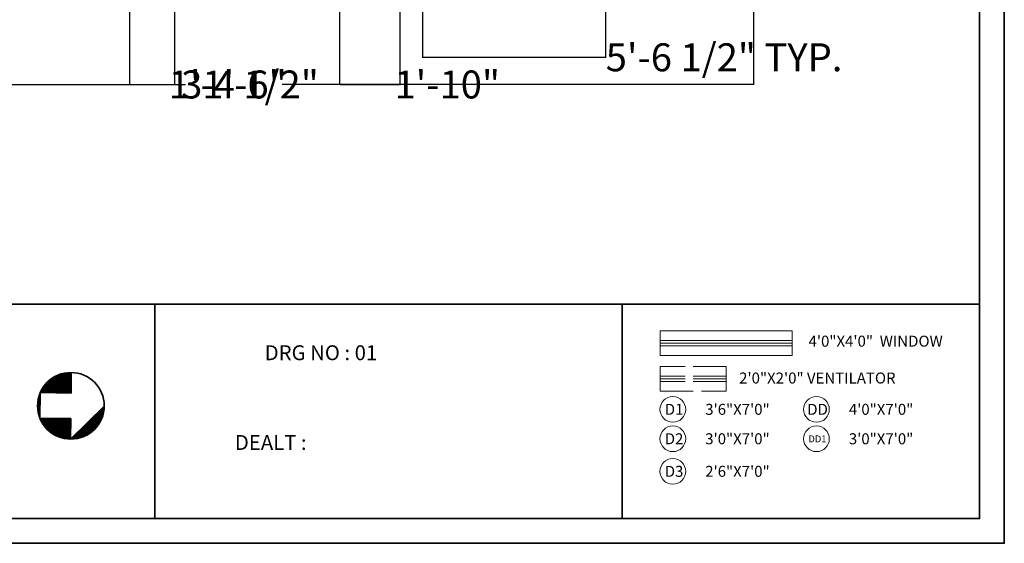
# Model space of a CAD drawing. Units: inches. Extents: x 1077 to 2505, y 1892 to 2728.
# Tile 20 of 26: x 2147 to 2505, y 1898 to 2089. Entities that reach past the tile are written whole.
import ezdxf

# ---------------------------------------------------------------- set-up
doc = ezdxf.new("R2010")
doc.units = ezdxf.units.IN
doc.linetypes.add('ACAD_ISO02W100', pattern=[15, 12, -3])
doc.layers.get('Defpoints').update_dxf_attribs({"color": 220, "linetype": 'ACAD_ISO02W100'})
for name, color, linetype, lineweight in [('A-ANNO-DIMS', 2, 'Continuous', 18), ('A-ANNO-LEGD', 7, 'Continuous', 13), ('A-ANNO-SYMB', 18, 'Continuous', 18), ('A-ANNO-TTLB', 7, 'Continuous', 35), ('A-GLAZ-VENT', 6, 'ACAD_ISO02W100', 13), ('A_TEXT_SMALL', 18, 'Continuous', 13), ('walls', 250, 'Continuous', 35), ('WINDOW', 160, 'Continuous', 13)]:
    doc.layers.add(name, color=color, linetype=linetype, lineweight=lineweight)
doc.styles.add('1-100DIM', font='txt', dxfattribs={"height": 0.3})
doc.styles.get("Standard").update_dxf_attribs({"font": 'arial.ttf'})
doc.dimstyles.get("Standard").update_dxf_attribs({"dimtxt": 10.18, "dimasz": 0.18, "dimexe": 0.18, "dimexo": 0.0625, "dimgap": 0.09, "dimtad": 0, "dimtih": 1, "dimtoh": 1, "dimdec": 0, "dimzin": 0, "dimdsep": 46, "dimlunit": 3, "dimtxsty": 'Standard', "dimcen": 0.09, "dimadec": 0, "dimazin": 0, "dimtfac": 1, "dimtdec": 0, "dimtofl": 0, "dimtmove": 0, "dimatfit": 3, "dimfxl": 1, "dimtolj": 1, "dimtzin": 0, "dimarcsym": 0})

# ---------------------------------------------------------------- blocks, each defined once
blk = doc.blocks.new('NORTH')
at = {"layer": 'walls'}
h = blk.add_hatch(dxfattribs=at)
h.set_pattern_fill('ANSI31', color=256, scale=6.087211)
h.set_pattern_definition([(45, (-41048.0969, 128612.4242), (-0.53803848, 0.53803848), [])])
h.paths.add_polyline_path([(6704.42, -25696.22), (6687.22, -25696.22, 0.302843), (6704.42, -25722.01)])
h.paths.add_polyline_path([(6743.1, -25696.22), (6725.9, -25696.22), (6725.9, -25722.01, 0.302843)])
h.paths.add_polyline_path([(6715.16, -25668.28), (6743.1, -25696.22, 0.414214)])
h.paths.add_polyline_path([(6725.9, -25722.01), (6704.42, -25722.01, 0.199872)])
for p, q in [((6743.1, -25696.22, 0.29), (6715.16, -25668.28, 0.29)), ((6687.22, -25696.22, 0.29), (6704.42, -25696.22, 0.29)), ((6704.42, -25722.01, 0.29), (6704.42, -25696.22, 0.29)), ((6725.9, -25722.01, 0.29), (6725.9, -25696.22, 0.29)), ((6725.9, -25696.22, 0.29), (6743.1, -25696.22, 0.29)), ((6704.42, -25722.01, 0.29), (6725.9, -25722.01, 0.29))]:
    blk.add_line(p, q, dxfattribs=at)
blk.add_circle((6715.16, -25696.22, 0.29), 27.94, dxfattribs=at)
blk = doc.blocks.new('WINDOW-48-EXT')
for p, q in [((0, 48), (0, 0)), ((3.5, 48), (3.5, 0)), ((4.5, 48), (4.5, 0)), ((5.5, 48), (5.5, 0)), ((9, 0), (9, 48))]:
    blk.add_line(p, q)
blk = doc.blocks.new('VENT-24')
for p, q in [((3.5, 24), (3.5, 0)), ((4.5, 24), (4.5, 0)), ((5.5, 24), (5.5, 0))]:
    blk.add_line(p, q)
blk.add_lwpolyline([(0, 0), (9, 0), (9, 24), (0, 24)], close=True)
blk = doc.blocks.new('SHEET-FRAME-RESIDENTIAL')
for p, q in [((9, 87.01), (534.52, 87.01)), ((234.45, 87.01), (234.45, 9)), ((404.52, 9), (404.52, 87.01))]:
    blk.add_line(p, q)
for points in [[(0, 830.04), (543.52, 830.04), (543.52, 0), (0, 0)], [(9, 821.04), (534.52, 821.04), (534.52, 9), (9, 9)]]:
    blk.add_lwpolyline(points, close=True)
blk = doc.blocks.new('*D57')
at = {"layer": 'A-ANNO-DIMS', "color": 0, "lineweight": -2, "transparency": 16777216}
for p, q in [((2293.39, 2099.33), (2293.39, 2075.01)), ((2359.99, 2099.33), (2359.99, 2075.01)), ((2293.57, 2075.19), (2359.81, 2075.19)), ((2359.99, 2075.19), (2360.17, 2075.19))]:
    blk.add_line(p, q, dxfattribs=at)
at = {"layer": 'A-ANNO-DIMS', "color": 0, "transparency": 16777216}
for points in [[(2293.57, 2075.22), (2293.57, 2075.16), (2293.39, 2075.19)], [(2359.81, 2075.22), (2359.81, 2075.16), (2359.99, 2075.19)]]:
    blk.add_solid(points, dxfattribs=at)
at = {"layer": 'Defpoints', "color": 0, "transparency": 16777216}
for p in [(2293.39, 2099.39), (2359.99, 2099.39), (2359.99, 2075.19)]:
    blk.add_point(p, dxfattribs=at)
at = {"layer": 'A-ANNO-DIMS', "color": 0, "transparency": 16777216, "insert": (2403.15, 2075.19), "char_height": 10.18, "attachment_point": 5}
blk.add_mtext('\\A1;5\'-6 1/2" TYP.', dxfattribs=at)
blk = doc.blocks.new('*D63')
at = {"layer": 'A-ANNO-DIMS', "color": 0, "lineweight": -2, "transparency": 16777216}
for p, q in [((2035.85, 2094.07), (2035.85, 2065.11)), ((2413.85, 2094.07), (2413.85, 2065.11)), ((2036.03, 2065.29), (2207.27, 2065.29)), ((2413.67, 2065.29), (2242.42, 2065.29))]:
    blk.add_line(p, q, dxfattribs=at)
at = {"layer": 'A-ANNO-DIMS', "color": 0, "transparency": 16777216}
for points in [[(2036.03, 2065.32), (2036.03, 2065.26), (2035.85, 2065.29)], [(2413.67, 2065.32), (2413.67, 2065.26), (2413.85, 2065.29)]]:
    blk.add_solid(points, dxfattribs=at)
at = {"layer": 'Defpoints', "color": 0, "transparency": 16777216}
for p in [(2035.85, 2094.14), (2413.85, 2094.14), (2413.85, 2065.29)]:
    blk.add_point(p, dxfattribs=at)
at = {"layer": 'A-ANNO-DIMS', "color": 0, "transparency": 16777216, "insert": (2224.85, 2065.29), "char_height": 10.18, "attachment_point": 5}
blk.add_mtext('\\A1;31\'-6"', dxfattribs=at)
blk = doc.blocks.new('*D69')
at = {"layer": 'A-ANNO-DIMS', "color": 0, "lineweight": -2, "transparency": 16777216}
for p, q in [((2263.27, 2262.49), (2263.27, 2065.11)), ((2285.18, 2262.49), (2285.18, 2065.11)), ((2263.45, 2065.29), (2285, 2065.29)), ((2285.18, 2065.29), (2285.36, 2065.29))]:
    blk.add_line(p, q, dxfattribs=at)
at = {"layer": 'A-ANNO-DIMS', "color": 0, "transparency": 16777216}
for points in [[(2263.45, 2065.32), (2263.45, 2065.26), (2263.27, 2065.29)], [(2285, 2065.32), (2285, 2065.26), (2285.18, 2065.29)]]:
    blk.add_solid(points, dxfattribs=at)
at = {"layer": 'Defpoints', "color": 0, "transparency": 16777216}
for p in [(2263.27, 2262.55), (2285.18, 2262.55), (2285.18, 2065.29)]:
    blk.add_point(p, dxfattribs=at)
at = {"layer": 'A-ANNO-DIMS', "color": 0, "transparency": 16777216, "insert": (2302.45, 2065.29), "char_height": 10.18, "attachment_point": 5}
blk.add_mtext('\\A1;1\'-10"', dxfattribs=at)
blk = doc.blocks.new('*D71')
at = {"layer": 'A-ANNO-DIMS', "color": 0, "lineweight": -2, "transparency": 16777216}
for p, q in [((2186.85, 2203.07), (2186.85, 2065.11)), ((2203.23, 2206.41), (2203.23, 2065.11)), ((2187.03, 2065.29), (2203.05, 2065.29)), ((2203.23, 2065.29), (2203.41, 2065.29))]:
    blk.add_line(p, q, dxfattribs=at)
at = {"layer": 'A-ANNO-DIMS', "color": 0, "transparency": 16777216}
for points in [[(2187.03, 2065.32), (2187.03, 2065.26), (2186.85, 2065.29)], [(2203.05, 2065.32), (2203.05, 2065.26), (2203.23, 2065.29)]]:
    blk.add_solid(points, dxfattribs=at)
at = {"layer": 'Defpoints', "color": 0, "transparency": 16777216}
for p in [(2203.23, 2206.48), (2186.85, 2203.14), (2203.23, 2065.29)]:
    blk.add_point(p, dxfattribs=at)
at = {"layer": 'A-ANNO-DIMS', "color": 0, "transparency": 16777216, "insert": (2228.41, 2065.29), "char_height": 10.18, "attachment_point": 5}
blk.add_mtext('\\A1;1\'-4 1/2"', dxfattribs=at)

msp = doc.modelspace()

# ---------------------------------------------------------------- linework, layer by layer
at = {"layer": 'A-ANNO-LEGD'}
for centre in [(2384.51, 1947.01), (2436.77, 1947.01), (2384.51, 1936.3), (2436.77, 1936.3), (2384.51, 1924.44)]:
    msp.add_circle(centre, 4.67, dxfattribs=at)
at = {"layer": 'WINDOW'}
for p, q in [((2379.94, 1975.6), (2379.94, 1966.6)), ((2427.94, 1975.6), (2427.94, 1966.6))]:
    msp.add_line(p, q, dxfattribs=at)

# ---------------------------------------------------------------- block references
at = {"layer": 'A-ANNO-SYMB', "xscale": 0.4341621291417894, "yscale": 0.4341621291417894, "zscale": 0.4341621291417894, "rotation": 269.2509902977627}
msp.add_blockref('NORTH', (13359.01, 4717.69, -0.13), dxfattribs=at)
at = {"layer": 'A-ANNO-TTLB'}
msp.add_blockref('SHEET-FRAME-RESIDENTIAL', (1961.57, 1898.25), dxfattribs=at)
at = {"layer": 'A-GLAZ-VENT', "rotation": 269.9999999999973}
msp.add_blockref('VENT-24', (2379.94, 1962.65), dxfattribs=at)
at = {"layer": 'WINDOW', "rotation": 90.00000000000087}
msp.add_blockref('WINDOW-48-EXT', (2427.94, 1966.6), dxfattribs=at)

# ---------------------------------------------------------------- texts
at = {"layer": 'A-ANNO-LEGD', "attachment_point": 1}
for s, width, insert, char_height in [('4\'0"X4\'0"  WINDOW', 55.3456, (2433.88, 1973.85), 4), ('2\'0"X2\'0" VENTILATOR', 67.3186, (2408.63, 1960.43), 4), ('D1', 8.4888, (2381.57, 1949.03), 4), ('3\'6"X7\'0"', 8.4888, (2396.29, 1949.03), 4), ('DD', 8.4888, (2433.41, 1949.03), 4), ('4\'0"X7\'0"', 8.4888, (2448.54, 1949.03), 4), ('D2', 8.4888, (2381.57, 1938.31), 4), ('3\'0"X7\'0"', 8.4888, (2396.29, 1938.31), 4), ('3\'0"X7\'0"', 8.4888, (2448.54, 1938.31), 4), ('DD1', 8.4888, (2433.82, 1937.53), 2.5), ('D3', 8.4888, (2381.57, 1926.46), 4), ('2\'6"X7\'0"', 8.4888, (2396.29, 1926.46), 4)]:
    msp.add_mtext_dynamic_manual_height_columns(s, width=width, gutter_width=12.5, heights=[0], dxfattribs=dict(at, insert=insert, char_height=char_height))
at = {"layer": 'A_TEXT_SMALL', "char_height": 5.4184, "attachment_point": 1, "style": '1-100DIM'}
for s, insert in [('{\\f@Malgun Gothic|b0|i0|c0|p34;DRG NO : 01}', (2236.04, 1970.34)), ('{\\f@Malgun Gothic|b0|i0|c0|p34;DEALT :}', (2225.19, 1937.68))]:
    msp.add_mtext_dynamic_manual_height_columns(s, width=152.9967, gutter_width=8.47, heights=[0], dxfattribs=dict(at, insert=insert))

# ---------------------------------------------------------------- dimensions: what is measured, and where the dimension line sits
at = {"layer": 'A-ANNO-DIMS'}
for base, p1, p2, picture, middle in [((2285.18, 2065.29), (2263.27, 2262.55), (2285.18, 2262.55), '*D69', (2302.45, 2065.29)), ((2203.23, 2065.29), (2186.85, 2203.14), (2203.23, 2206.48), '*D71', (2228.41, 2065.29)), ((2413.85, 2065.29), (2035.85, 2094.14), (2413.85, 2094.14), '*D63', (2224.85, 2065.29))]:
    dim = msp.add_linear_dim(base=base, p1=p1, p2=p2, dimstyle='Standard', override={"dimdec": 1, "dimlfac": 1, "dimrnd": 0, "dimzin": 1, "dimdsep": 46, "dimlunit": 4, "dimfrac": 2}, dxfattribs=at)
    dim.commit()
    dim.dimension.update_dxf_attribs({"geometry": picture, "text_midpoint": middle})
dim = msp.add_linear_dim(base=(2359.99, 2075.19), p1=(2293.39, 2099.39), p2=(2359.99, 2099.39), text='<> TYP.', dimstyle='Standard', override={"dimdec": 1, "dimlfac": 1, "dimrnd": 0, "dimzin": 1, "dimdsep": 46, "dimlunit": 4, "dimfrac": 2}, dxfattribs=at)
dim.commit()
dim.dimension.update_dxf_attribs({"geometry": '*D57', "text_midpoint": (2403.15, 2075.19)})

doc.saveas('drawing.dxf')
